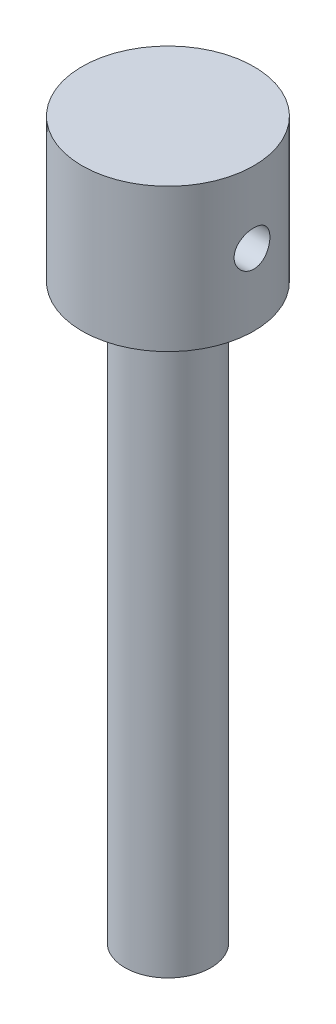
ISO-10303-21;
HEADER;
FILE_DESCRIPTION(('STEP AP214'),'2;1');
FILE_NAME('part.step','',(''),(''),'','','');
FILE_SCHEMA(('AUTOMOTIVE_DESIGN { 1 0 10303 214 1 1 1 1 }'));
ENDSEC;
DATA;
#1=APPLICATION_CONTEXT('core data for automotive mechanical design processes');
#2=APPLICATION_PROTOCOL_DEFINITION('international standard','automotive_design',2000,#1);
#3=PRODUCT_CONTEXT('',#1,'mechanical');
#4=PRODUCT('Part','Part','',(#3));
#5=PRODUCT_RELATED_PRODUCT_CATEGORY('part','',(#4));
#6=PRODUCT_DEFINITION_FORMATION('','',#4);
#7=PRODUCT_DEFINITION_CONTEXT('part definition',#1,'design');
#8=PRODUCT_DEFINITION('design','',#6,#7);
#9=PRODUCT_DEFINITION_SHAPE('','',#8);
#10=(LENGTH_UNIT() NAMED_UNIT(*) SI_UNIT(.MILLI.,.METRE.));
#11=(NAMED_UNIT(*) PLANE_ANGLE_UNIT() SI_UNIT($,.RADIAN.));
#12=(NAMED_UNIT(*) SI_UNIT($,.STERADIAN.) SOLID_ANGLE_UNIT());
#13=UNCERTAINTY_MEASURE_WITH_UNIT(LENGTH_MEASURE(1.E-05),#10,'distance_accuracy_value','');
#14=(GEOMETRIC_REPRESENTATION_CONTEXT(3) GLOBAL_UNCERTAINTY_ASSIGNED_CONTEXT((#13)) GLOBAL_UNIT_ASSIGNED_CONTEXT((#10,
#11,#12)) REPRESENTATION_CONTEXT('',''));
#15=CARTESIAN_POINT('',(0.,0.,0.));
#16=DIRECTION('',(0.,0.,1.));
#17=DIRECTION('',(1.,0.,0.));
#18=AXIS2_PLACEMENT_3D('',#15,#16,#17);
#19=CARTESIAN_POINT('',(0.,80.,0.));
#20=DIRECTION('',(0.,-1.,0.));
#21=DIRECTION('',(0.,0.,-1.));
#22=AXIS2_PLACEMENT_3D('',#19,#20,#21);
#23=CYLINDRICAL_SURFACE('',#22,6.);
#24=CARTESIAN_POINT('',(0.,80.,0.));
#25=DIRECTION('',(0.,1.,0.));
#26=DIRECTION('',(0.,0.,1.));
#27=AXIS2_PLACEMENT_3D('',#24,#25,#26);
#28=CIRCLE('',#27,6.);
#29=CARTESIAN_POINT('',(0.,80.,6.));
#30=VERTEX_POINT('',#29);
#31=EDGE_CURVE('E10',#30,#30,#28,.T.);
#32=ORIENTED_EDGE('',*,*,#31,.F.);
#33=EDGE_LOOP('',(#32));
#34=FACE_BOUND('',#33,.T.);
#35=CARTESIAN_POINT('',(0.,0.,0.));
#36=DIRECTION('',(0.,1.,0.));
#37=DIRECTION('',(0.,0.,1.));
#38=AXIS2_PLACEMENT_3D('',#35,#36,#37);
#39=CIRCLE('',#38,6.);
#40=CARTESIAN_POINT('',(0.,0.,6.));
#41=VERTEX_POINT('',#40);
#42=EDGE_CURVE('E47',#41,#41,#39,.T.);
#43=ORIENTED_EDGE('',*,*,#42,.T.);
#44=EDGE_LOOP('',(#43));
#45=FACE_BOUND('',#44,.T.);
#46=ADVANCED_FACE('F40',(#34,#45),#23,.T.);
#47=CARTESIAN_POINT('',(0.,0.,0.));
#48=DIRECTION('',(0.,1.,0.));
#49=DIRECTION('',(0.,0.,1.));
#50=AXIS2_PLACEMENT_3D('',#47,#48,#49);
#51=PLANE('',#50);
#52=ORIENTED_EDGE('',*,*,#42,.F.);
#53=EDGE_LOOP('',(#52));
#54=FACE_BOUND('',#53,.T.);
#55=ADVANCED_FACE('F85',(#54),#51,.F.);
#56=CARTESIAN_POINT('',(0.,100.,0.));
#57=DIRECTION('',(0.,-1.,0.));
#58=DIRECTION('',(0.,0.,-1.));
#59=AXIS2_PLACEMENT_3D('',#56,#57,#58);
#60=CYLINDRICAL_SURFACE('',#59,12.);
#61=CARTESIAN_POINT('',(-11.7366945943055,90.,-2.5));
#62=CARTESIAN_POINT('',(-11.7366973843002,90.1387812303038,-2.499995017553));
#63=CARTESIAN_POINT('',(-11.7391829184982,90.2776239440309,-2.48840458867923));
#64=CARTESIAN_POINT('',(-11.7488403116286,90.551372634634,-2.44239298467531));
#65=CARTESIAN_POINT('',(-11.7560157627658,90.6862755110127,-2.40795430880677));
#66=CARTESIAN_POINT('',(-11.7742058592406,90.9481447456699,-2.31736795014468));
#67=CARTESIAN_POINT('',(-11.7852165141394,91.0751191919836,-2.26124282497867));
#68=CARTESIAN_POINT('',(-11.8098316267143,91.3178489992912,-2.12893977203463));
#69=CARTESIAN_POINT('',(-11.8234359795523,91.43360481346,-2.05276265471639));
#70=CARTESIAN_POINT('',(-11.8519386932295,91.6523907503069,-1.88127279893218));
#71=CARTESIAN_POINT('',(-11.8668522874608,91.7552237872529,-1.78571110973935));
#72=CARTESIAN_POINT('',(-11.8961593360515,91.9435221372962,-1.57870244776128));
#73=CARTESIAN_POINT('',(-11.9105527521983,92.0289861765829,-1.46725431091201));
#74=CARTESIAN_POINT('',(-11.937362702377,92.1808917761657,-1.23032410599918));
#75=CARTESIAN_POINT('',(-11.9497591726249,92.2471450529265,-1.10471885640989));
#76=CARTESIAN_POINT('',(-11.971006946866,92.3575321057196,-0.843857102013447));
#77=CARTESIAN_POINT('',(-11.9798586112245,92.4016681303071,-0.708601579901191));
#78=CARTESIAN_POINT('',(-11.9929117978436,92.465951522235,-0.434325808401013));
#79=CARTESIAN_POINT('',(-11.9971778391985,92.4864320343903,-0.295386761832723));
#80=CARTESIAN_POINT('',(-12.0008022516122,92.5038633915141,-0.015983697679055));
#81=CARTESIAN_POINT('',(-12.0001611340738,92.5008166883862,0.124480159473672));
#82=CARTESIAN_POINT('',(-11.9940931618102,92.4715307980865,0.40065317239914));
#83=CARTESIAN_POINT('',(-11.9887403791317,92.4456505620838,0.536402257452946));
#84=CARTESIAN_POINT('',(-11.9739344179777,92.3720027493374,0.801587492579501));
#85=CARTESIAN_POINT('',(-11.9644810658381,92.3242342455939,0.931023375022041));
#86=CARTESIAN_POINT('',(-11.9424153464785,92.207839895749,1.18092001076937));
#87=CARTESIAN_POINT('',(-11.9297820825069,92.1390754115807,1.3013142699633));
#88=CARTESIAN_POINT('',(-11.9027460088038,91.9827439943192,1.52898691302129));
#89=CARTESIAN_POINT('',(-11.8883429791665,91.8951747235878,1.63626366363284));
#90=CARTESIAN_POINT('',(-11.8590340046655,91.7017567502179,1.83678840655382));
#91=CARTESIAN_POINT('',(-11.8441236995185,91.5955938800361,1.92973297498959));
#92=CARTESIAN_POINT('',(-11.8157374529799,91.3690359020104,2.09655194480976));
#93=CARTESIAN_POINT('',(-11.8022615435432,91.2486404772255,2.1704259213996));
#94=CARTESIAN_POINT('',(-11.7782599681831,90.9965754903424,2.29712434276909));
#95=CARTESIAN_POINT('',(-11.7677417046425,90.8648786986131,2.34989610979454));
#96=CARTESIAN_POINT('',(-11.7509521282072,90.5942167612612,2.43247155077345));
#97=CARTESIAN_POINT('',(-11.7446802101436,90.4552526543838,2.46227849764697));
#98=CARTESIAN_POINT('',(-11.7372156647826,90.1767605873622,2.49761727734035));
#99=CARTESIAN_POINT('',(-11.7359310372695,90.037290830926,2.50358885835997));
#100=CARTESIAN_POINT('',(-11.7383390403741,89.7593483769197,2.49227386878589));
#101=CARTESIAN_POINT('',(-11.7420313630525,89.6208756181954,2.47498873715726));
#102=CARTESIAN_POINT('',(-11.7538907645233,89.3503589678838,2.41803116650968));
#103=CARTESIAN_POINT('',(-11.76201022566,89.2182626656424,2.37859682753743));
#104=CARTESIAN_POINT('',(-11.7817667700624,88.9625520211168,2.27871621721839));
#105=CARTESIAN_POINT('',(-11.7934041638211,88.8389384286992,2.21826809112293));
#106=CARTESIAN_POINT('',(-11.8190900387438,88.6017871175676,2.07709196362969));
#107=CARTESIAN_POINT('',(-11.8331701329665,88.4884155910677,1.99609065470792));
#108=CARTESIAN_POINT('',(-11.8620696798782,88.2767135016899,1.81646888113976));
#109=CARTESIAN_POINT('',(-11.8768892153306,88.1783846275216,1.71784644101034));
#110=CARTESIAN_POINT('',(-11.9058984863347,87.9978745738057,1.50380090168668));
#111=CARTESIAN_POINT('',(-11.9200734943982,87.9159918099472,1.3881238152291));
#112=CARTESIAN_POINT('',(-11.9459341754481,87.772822495824,1.14440020443272));
#113=CARTESIAN_POINT('',(-11.9576199584164,87.7115350355251,1.01635422695377));
#114=CARTESIAN_POINT('',(-11.9771229654136,87.6117226413653,0.752284235695843));
#115=CARTESIAN_POINT('',(-11.9849632627299,87.5730616689113,0.616313421940395));
#116=CARTESIAN_POINT('',(-11.9959912282046,87.5191711919838,0.339626801006947));
#117=CARTESIAN_POINT('',(-11.9991795068579,87.5039386129345,0.198911618923388));
#118=CARTESIAN_POINT('',(-12.0005281611387,87.497464755903,-0.0804266869406707));
#119=CARTESIAN_POINT('',(-11.9987822750957,87.5057762000105,-0.219039184355822));
#120=CARTESIAN_POINT('',(-11.99065748189,87.5451612773059,-0.492845740747129));
#121=CARTESIAN_POINT('',(-11.9842786434588,87.5762345728137,-0.62803985040549));
#122=CARTESIAN_POINT('',(-11.9676092015489,87.660055589297,-0.890863930984021));
#123=CARTESIAN_POINT('',(-11.9573290681437,87.7127453277057,-1.01851310000873));
#124=CARTESIAN_POINT('',(-11.9339599069615,87.8382447954646,-1.2632211344418));
#125=CARTESIAN_POINT('',(-11.9208706346327,87.9110562766883,-1.38027907656019));
#126=CARTESIAN_POINT('',(-11.8930319356995,88.0762193359845,-1.60268064259534));
#127=CARTESIAN_POINT('',(-11.8782576059507,88.1688885761055,-1.70778526722739));
#128=CARTESIAN_POINT('',(-11.8488557363333,88.3704890020021,-1.90110548396524));
#129=CARTESIAN_POINT('',(-11.8342282323044,88.4794240599264,-1.98931704315915));
#130=CARTESIAN_POINT('',(-11.8065838324643,88.712018204841,-2.14734903704122));
#131=CARTESIAN_POINT('',(-11.7935881325424,88.8358368228206,-2.21693856248136));
#132=CARTESIAN_POINT('',(-11.7709407916825,89.0936503120622,-2.3342125584477));
#133=CARTESIAN_POINT('',(-11.7612862067076,89.2276360968785,-2.381916325835));
#134=CARTESIAN_POINT('',(-11.7482800883641,89.4682125631532,-2.44513108264677));
#135=CARTESIAN_POINT('',(-11.7439632719021,89.5734590731905,-2.46566898011599));
#136=CARTESIAN_POINT('',(-11.7381695052653,89.7857915610376,-2.4931050871655));
#137=CARTESIAN_POINT('',(-11.7366924407628,89.8928774646188,-2.50000384585405));
#138=CARTESIAN_POINT('',(-11.7366945943055,90.,-2.5));
#139=B_SPLINE_CURVE_WITH_KNOTS('',3,(#61,#62,#63,#64,#65,#66,#67,#68,#69,#70,#71,#72,#73,#74,
#75,#76,#77,#78,#79,#80,#81,#82,#83,#84,#85,#86,#87,#88,#89,#90,#91,#92,#93,#94,#95,#96,#97,#98,
#99,#100,#101,#102,#103,#104,#105,#106,#107,#108,#109,#110,#111,#112,#113,#114,#115,#116,#117,
#118,#119,#120,#121,#122,#123,#124,#125,#126,#127,#128,#129,#130,#131,#132,#133,#134,#135,#136,
#137,#138),.UNSPECIFIED.,.T.,.F.,(4,2,2,2,2,2,2,2,2,2,2,2,2,2,2,2,2,2,2,2,2,2,2,2,2,2,2,2,2,2,2,
2,2,2,2,2,2,2,4),(0.,0.415951308142525,0.83222158483494,1.24806002960546,1.66388166963158,
2.08542666935768,2.50700257327748,2.93258052533687,3.35811520213866,3.77758097718529,
4.19700303792678,4.60994682832923,5.02290810911741,5.43865743955899,5.8544584820852,
6.27811724489827,6.70178544383257,7.12650474664976,7.55116350775194,7.96795032019584,
8.38471134593048,8.79707572463845,9.20947650928063,9.62767835869304,10.0459271216437,
10.4711891750669,10.8964324351808,11.3190919929707,11.7416960791916,12.1563258784529,
12.5709495266596,12.984468211702,13.3980229105635,13.8187663795715,14.2396101685507,
14.6654530271772,15.0909196914727,15.4119973517483,15.7330620852562),.UNSPECIFIED.);
#140=CARTESIAN_POINT('',(-11.7366945943055,90.,-2.5));
#141=VERTEX_POINT('',#140);
#142=EDGE_CURVE('E37',#141,#141,#139,.T.);
#143=ORIENTED_EDGE('',*,*,#142,.T.);
#144=EDGE_LOOP('',(#143));
#145=FACE_BOUND('',#144,.T.);
#146=CARTESIAN_POINT('',(11.7366945943055,90.,-2.5));
#147=CARTESIAN_POINT('',(11.7366973843002,89.8612187696963,-2.499995017553));
#148=CARTESIAN_POINT('',(11.7391829184982,89.7223760559691,-2.48840458867923));
#149=CARTESIAN_POINT('',(11.7488403116286,89.448627365366,-2.44239298467531));
#150=CARTESIAN_POINT('',(11.7560157627658,89.3137244889873,-2.40795430880677));
#151=CARTESIAN_POINT('',(11.7742058592406,89.0518552543301,-2.31736795014468));
#152=CARTESIAN_POINT('',(11.7852165141394,88.9248808080164,-2.26124282497867));
#153=CARTESIAN_POINT('',(11.8098316267143,88.6821510007088,-2.12893977203463));
#154=CARTESIAN_POINT('',(11.8234359795523,88.56639518654,-2.05276265471639));
#155=CARTESIAN_POINT('',(11.8519386932295,88.3476092496931,-1.88127279893218));
#156=CARTESIAN_POINT('',(11.8668522874608,88.2447762127471,-1.78571110973934));
#157=CARTESIAN_POINT('',(11.8961593360515,88.0564778627038,-1.57870244776127));
#158=CARTESIAN_POINT('',(11.9105527521983,87.9710138234171,-1.467254310912));
#159=CARTESIAN_POINT('',(11.937362702377,87.8191082238343,-1.23032410599918));
#160=CARTESIAN_POINT('',(11.9497591726249,87.7528549470735,-1.10471885640988));
#161=CARTESIAN_POINT('',(11.971006946866,87.6424678942805,-0.84385710201344));
#162=CARTESIAN_POINT('',(11.9798586112245,87.5983318696929,-0.708601579901187));
#163=CARTESIAN_POINT('',(11.9929117978436,87.5340484777651,-0.434325808401013));
#164=CARTESIAN_POINT('',(11.9971778391985,87.5135679656097,-0.295386761832722));
#165=CARTESIAN_POINT('',(12.0008022516122,87.496136608486,-0.0159836976790537));
#166=CARTESIAN_POINT('',(12.0001611340738,87.4991833116138,0.124480159473673));
#167=CARTESIAN_POINT('',(11.9940931618102,87.5284692019135,0.40065317239914));
#168=CARTESIAN_POINT('',(11.9887403791317,87.5543494379162,0.536402257452946));
#169=CARTESIAN_POINT('',(11.9739344179777,87.6279972506626,0.801587492579501));
#170=CARTESIAN_POINT('',(11.9644810658381,87.6757657544062,0.931023375022041));
#171=CARTESIAN_POINT('',(11.9424153464785,87.792160104251,1.18092001076937));
#172=CARTESIAN_POINT('',(11.9297820825069,87.8609245884193,1.3013142699633));
#173=CARTESIAN_POINT('',(11.9027460088038,88.0172560056808,1.52898691302129));
#174=CARTESIAN_POINT('',(11.8883429791665,88.1048252764123,1.63626366363284));
#175=CARTESIAN_POINT('',(11.8590340046655,88.2982432497821,1.83678840655382));
#176=CARTESIAN_POINT('',(11.8441236995185,88.4044061199639,1.92973297498959));
#177=CARTESIAN_POINT('',(11.8157374529799,88.6309640979896,2.09655194480976));
#178=CARTESIAN_POINT('',(11.8022615435432,88.7513595227745,2.1704259213996));
#179=CARTESIAN_POINT('',(11.7782599681831,89.0034245096576,2.29712434276909));
#180=CARTESIAN_POINT('',(11.7677417046425,89.1351213013869,2.34989610979454));
#181=CARTESIAN_POINT('',(11.7509521282072,89.4057832387388,2.43247155077345));
#182=CARTESIAN_POINT('',(11.7446802101436,89.5447473456162,2.46227849764697));
#183=CARTESIAN_POINT('',(11.7372156647826,89.8232394126378,2.49761727734035));
#184=CARTESIAN_POINT('',(11.7359310372695,89.9627091690741,2.50358885835997));
#185=CARTESIAN_POINT('',(11.7383390403741,90.2406516230803,2.49227386878589));
#186=CARTESIAN_POINT('',(11.7420313630525,90.3791243818047,2.47498873715726));
#187=CARTESIAN_POINT('',(11.7538907645233,90.6496410321163,2.41803116650968));
#188=CARTESIAN_POINT('',(11.76201022566,90.7817373343577,2.37859682753743));
#189=CARTESIAN_POINT('',(11.7817667700624,91.0374479788832,2.27871621721839));
#190=CARTESIAN_POINT('',(11.7934041638211,91.1610615713008,2.21826809112293));
#191=CARTESIAN_POINT('',(11.8190900387438,91.3982128824325,2.07709196362969));
#192=CARTESIAN_POINT('',(11.8331701329665,91.5115844089324,1.99609065470792));
#193=CARTESIAN_POINT('',(11.8620696798782,91.7232864983101,1.81646888113976));
#194=CARTESIAN_POINT('',(11.8768892153306,91.8216153724785,1.71784644101034));
#195=CARTESIAN_POINT('',(11.9058984863347,92.0021254261944,1.50380090168668));
#196=CARTESIAN_POINT('',(11.9200734943982,92.0840081900528,1.3881238152291));
#197=CARTESIAN_POINT('',(11.9459341754481,92.227177504176,1.14440020443272));
#198=CARTESIAN_POINT('',(11.9576199584164,92.2884649644749,1.01635422695376));
#199=CARTESIAN_POINT('',(11.9771229654136,92.3882773586347,0.752284235695844));
#200=CARTESIAN_POINT('',(11.9849632627299,92.4269383310887,0.616313421940395));
#201=CARTESIAN_POINT('',(11.9959912282046,92.4808288080162,0.339626801006947));
#202=CARTESIAN_POINT('',(11.9991795068579,92.4960613870655,0.198911618923388));
#203=CARTESIAN_POINT('',(12.0005281611387,92.502535244097,-0.0804266869406694));
#204=CARTESIAN_POINT('',(11.9987822750957,92.4942237999895,-0.219039184355819));
#205=CARTESIAN_POINT('',(11.99065748189,92.4548387226941,-0.492845740747126));
#206=CARTESIAN_POINT('',(11.9842786434588,92.4237654271863,-0.628039850405489));
#207=CARTESIAN_POINT('',(11.9676092015489,92.339944410703,-0.890863930984021));
#208=CARTESIAN_POINT('',(11.9573290681437,92.2872546722944,-1.01851310000873));
#209=CARTESIAN_POINT('',(11.9339599069615,92.1617552045355,-1.2632211344418));
#210=CARTESIAN_POINT('',(11.9208706346327,92.0889437233117,-1.38027907656019));
#211=CARTESIAN_POINT('',(11.8930319356995,91.9237806640155,-1.60268064259533));
#212=CARTESIAN_POINT('',(11.8782576059507,91.8311114238945,-1.70778526722738));
#213=CARTESIAN_POINT('',(11.8488557363333,91.6295109979979,-1.90110548396523));
#214=CARTESIAN_POINT('',(11.8342282323044,91.5205759400736,-1.98931704315914));
#215=CARTESIAN_POINT('',(11.8065838324643,91.287981795159,-2.14734903704122));
#216=CARTESIAN_POINT('',(11.7935881325424,91.1641631771794,-2.21693856248136));
#217=CARTESIAN_POINT('',(11.7709407916825,90.9063496879379,-2.3342125584477));
#218=CARTESIAN_POINT('',(11.7612862067076,90.7723639031215,-2.381916325835));
#219=CARTESIAN_POINT('',(11.7482800883641,90.5317874368468,-2.44513108264677));
#220=CARTESIAN_POINT('',(11.7439632719021,90.4265409268095,-2.46566898011599));
#221=CARTESIAN_POINT('',(11.7381695052653,90.2142084389624,-2.4931050871655));
#222=CARTESIAN_POINT('',(11.7366924407628,90.1071225353813,-2.50000384585405));
#223=CARTESIAN_POINT('',(11.7366945943055,90.,-2.5));
#224=B_SPLINE_CURVE_WITH_KNOTS('',3,(#146,#147,#148,#149,#150,#151,#152,#153,#154,#155,#156,
#157,#158,#159,#160,#161,#162,#163,#164,#165,#166,#167,#168,#169,#170,#171,#172,#173,#174,#175,
#176,#177,#178,#179,#180,#181,#182,#183,#184,#185,#186,#187,#188,#189,#190,#191,#192,#193,#194,
#195,#196,#197,#198,#199,#200,#201,#202,#203,#204,#205,#206,#207,#208,#209,#210,#211,#212,#213,
#214,#215,#216,#217,#218,#219,#220,#221,#222,#223),.UNSPECIFIED.,.T.,.F.,(4,2,2,2,2,2,2,2,2,2,2,
2,2,2,2,2,2,2,2,2,2,2,2,2,2,2,2,2,2,2,2,2,2,2,2,2,2,2,4),(0.,0.415951308142525,0.83222158483494,
1.24806002960546,1.66388166963158,2.08542666935771,2.50700257327748,2.93258052533688,
3.35811520213866,3.77758097718529,4.19700303792677,4.60994682832922,5.02290810911741,
5.43865743955899,5.8544584820852,6.27811724489827,6.70178544383257,7.12650474664976,
7.55116350775193,7.96795032019584,8.38471134593048,8.79707572463845,9.20947650928062,
9.62767835869304,10.0459271216437,10.4711891750669,10.8964324351808,11.3190919929707,
11.7416960791916,12.1563258784529,12.5709495266596,12.984468211702,13.3980229105635,
13.8187663795715,14.2396101685507,14.6654530271772,15.0909196914727,15.4119973517483,
15.7330620852562),.UNSPECIFIED.);
#225=CARTESIAN_POINT('',(11.7366945943055,90.,-2.5));
#226=VERTEX_POINT('',#225);
#227=EDGE_CURVE('E56',#226,#226,#224,.T.);
#228=ORIENTED_EDGE('',*,*,#227,.T.);
#229=EDGE_LOOP('',(#228));
#230=FACE_BOUND('',#229,.T.);
#231=CARTESIAN_POINT('',(0.,100.,0.));
#232=DIRECTION('',(0.,1.,0.));
#233=DIRECTION('',(0.,0.,1.));
#234=AXIS2_PLACEMENT_3D('',#231,#232,#233);
#235=CIRCLE('',#234,12.);
#236=CARTESIAN_POINT('',(0.,100.,12.));
#237=VERTEX_POINT('',#236);
#238=EDGE_CURVE('E53',#237,#237,#235,.T.);
#239=ORIENTED_EDGE('',*,*,#238,.F.);
#240=EDGE_LOOP('',(#239));
#241=FACE_BOUND('',#240,.T.);
#242=CARTESIAN_POINT('',(0.,80.,0.));
#243=DIRECTION('',(0.,1.,0.));
#244=DIRECTION('',(0.,0.,1.));
#245=AXIS2_PLACEMENT_3D('',#242,#243,#244);
#246=CIRCLE('',#245,12.);
#247=CARTESIAN_POINT('',(0.,80.,12.));
#248=VERTEX_POINT('',#247);
#249=EDGE_CURVE('E60',#248,#248,#246,.T.);
#250=ORIENTED_EDGE('',*,*,#249,.T.);
#251=EDGE_LOOP('',(#250));
#252=FACE_BOUND('',#251,.T.);
#253=ADVANCED_FACE('F64',(#145,#230,#241,#252),#60,.T.);
#254=CARTESIAN_POINT('',(0.,100.,0.));
#255=DIRECTION('',(0.,1.,0.));
#256=DIRECTION('',(0.,0.,1.));
#257=AXIS2_PLACEMENT_3D('',#254,#255,#256);
#258=PLANE('',#257);
#259=ORIENTED_EDGE('',*,*,#238,.T.);
#260=EDGE_LOOP('',(#259));
#261=FACE_BOUND('',#260,.T.);
#262=ADVANCED_FACE('F71',(#261),#258,.T.);
#263=CARTESIAN_POINT('',(0.,80.,0.));
#264=DIRECTION('',(0.,1.,0.));
#265=DIRECTION('',(0.,0.,1.));
#266=AXIS2_PLACEMENT_3D('',#263,#264,#265);
#267=PLANE('',#266);
#268=ORIENTED_EDGE('',*,*,#31,.T.);
#269=EDGE_LOOP('',(#268));
#270=FACE_BOUND('',#269,.T.);
#271=ORIENTED_EDGE('',*,*,#249,.F.);
#272=EDGE_LOOP('',(#271));
#273=FACE_BOUND('',#272,.T.);
#274=ADVANCED_FACE('F72',(#270,#273),#267,.F.);
#275=CARTESIAN_POINT('',(-25.,90.,0.));
#276=DIRECTION('',(1.,0.,0.));
#277=DIRECTION('',(0.,0.,-1.));
#278=AXIS2_PLACEMENT_3D('',#275,#276,#277);
#279=CYLINDRICAL_SURFACE('',#278,2.5);
#280=ORIENTED_EDGE('',*,*,#227,.F.);
#281=EDGE_LOOP('',(#280));
#282=FACE_BOUND('',#281,.T.);
#283=ORIENTED_EDGE('',*,*,#142,.F.);
#284=EDGE_LOOP('',(#283));
#285=FACE_BOUND('',#284,.T.);
#286=ADVANCED_FACE('F66',(#282,#285),#279,.F.);
#287=CLOSED_SHELL('',(#46,#55,#253,#262,#274,#286));
#288=MANIFOLD_SOLID_BREP('B2',#287);
#289=ADVANCED_BREP_SHAPE_REPRESENTATION('',(#18,#288),#14);
#290=SHAPE_DEFINITION_REPRESENTATION(#9,#289);
ENDSEC;
END-ISO-10303-21;
